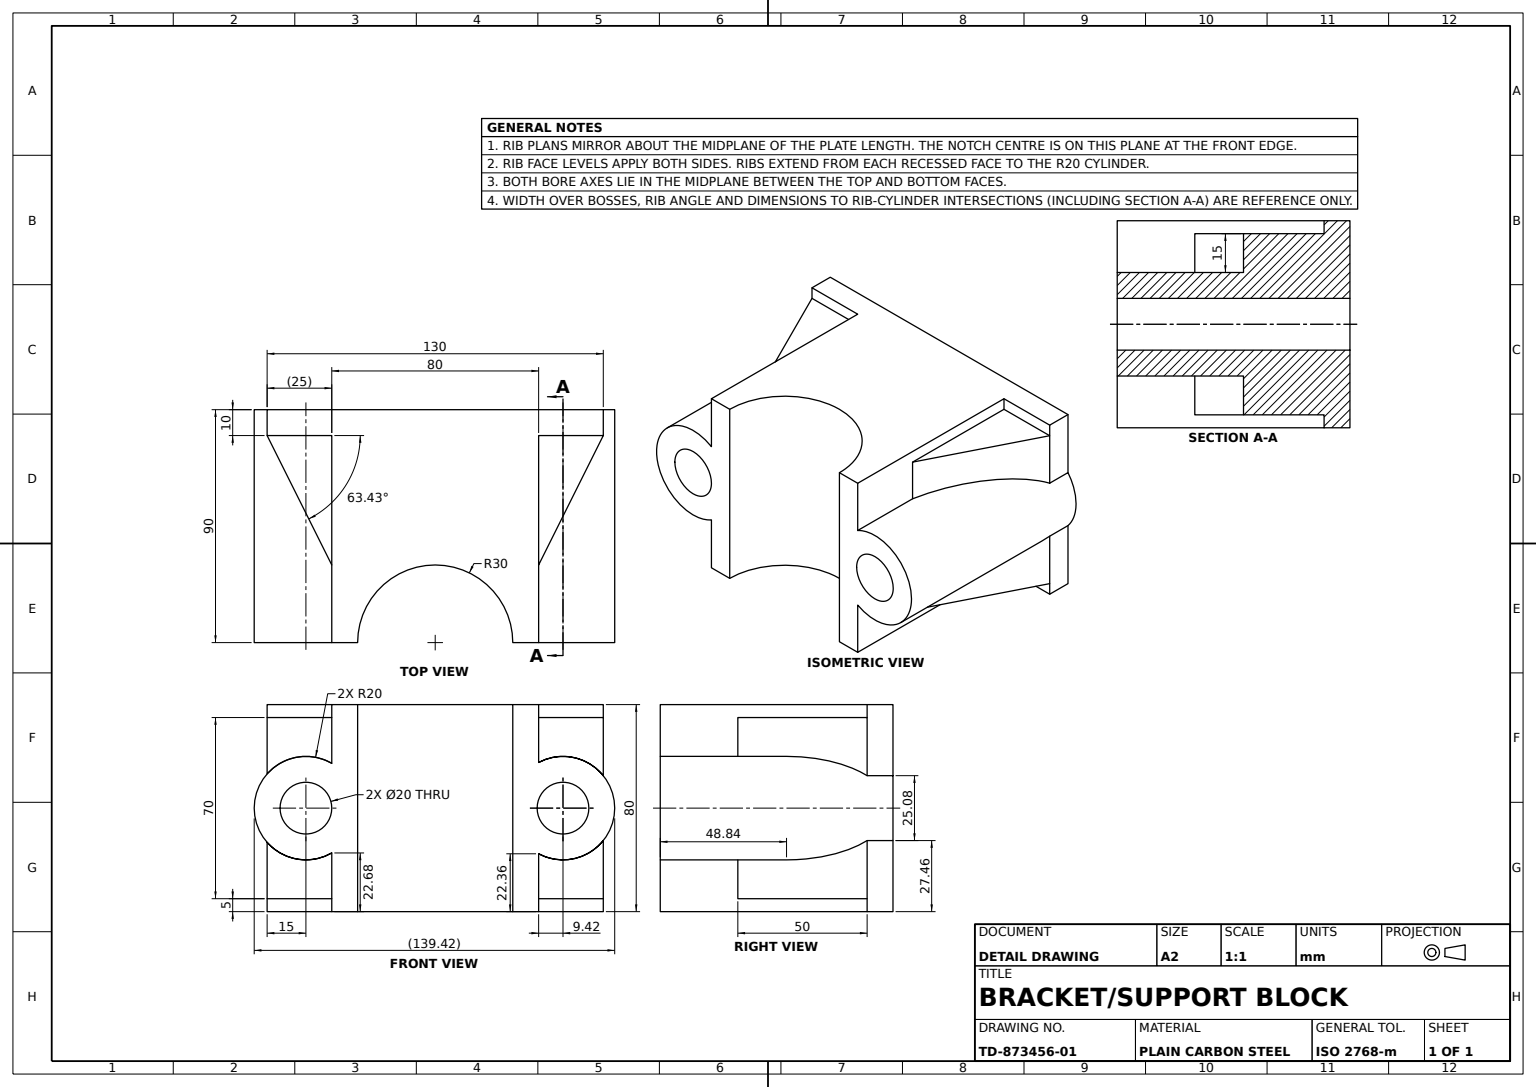
from build123d import *

# Parameters (mm, degrees)
BASE_PLATE_SKETCH_W    = 130
BASE_PLATE_SKETCH_H    = 80
BASE_PLATE_10MM_DEPTH  = 10
MAIN_BODY_PROFILE_W    = 10
MAIN_BODY_PROFILE_H    = 80
MAIN_BODY_DEPTH        = 80
SIDE_WALL_A_DEPTH      = 90
SIDE_WALL_B_DEPTH      = 90
HALF_BORE_SKETCH_R     = 10
HALF_BORE_CUT_DEPTH    = 90
RIB_A_DEPTH            = 28
RIB_B_DEPTH            = 28
BOSS_DEPTH             = 28
RECESS_CUT_A_5MM_DEPTH = 5
RECESS_CUT_B_5MM_DEPTH = 5


with BuildPart() as part:
    # Base Plate Sketch → Base Plate 10mm (new body)
    with BuildSketch(Plane.XY):
        with Locations((65, 40)):
            Rectangle(BASE_PLATE_SKETCH_W, BASE_PLATE_SKETCH_H)
    extrude(amount=BASE_PLATE_10MM_DEPTH)

    # Main Body Profile → Main Body (add)
    with BuildSketch(Plane.XZ):
        with Locations((30, 50)):
            Rectangle(MAIN_BODY_PROFILE_W, MAIN_BODY_PROFILE_H)
        with BuildLine():
            Line((35, 10), (65, 10))
            Line((65, 10), (95, 10))
            Line((95, 10), (95, 90))
            ThreePointArc((95, 90), (65, 60), (35, 90))
            Line((35, 90), (35, 10))
        make_face()
        with Locations((100, 50)):
            Rectangle(MAIN_BODY_PROFILE_W, MAIN_BODY_PROFILE_H)
    extrude(amount=-MAIN_BODY_DEPTH)

    # Side Wall A Sketch → Side Wall A (add)
    with BuildSketch(Plane.XY.offset(90)):
        with BuildLine():
            Line((105, 57.643408065), (105, 22.356591935))
            ThreePointArc((105, 22.356591935), (134.418606683, 40), (105, 57.643408065))
        make_face()
    extrude(amount=-SIDE_WALL_A_DEPTH)

    # Side Wall B Sketch → Side Wall B (add)
    with BuildSketch(Plane.XY.offset(90)):
        with BuildLine():
            Line((25, 57.320508076), (25, 22.679491924))
            ThreePointArc((25, 22.679491924), (-5, 40), (25, 57.320508076))
        make_face()
    extrude(amount=-SIDE_WALL_B_DEPTH)

    # Half Bore Sketch → Half Bore Cut (cut)
    with BuildSketch(Plane.XY.offset(90)):
        with Locations((114.418606683, 40)):
            Circle(HALF_BORE_SKETCH_R)
        with Locations((15, 40)):
            Circle(HALF_BORE_SKETCH_R)
    extrude(amount=-HALF_BORE_CUT_DEPTH, mode=Mode.SUBTRACT)

    # Rib A Sketch → Rib A (add)
    with BuildSketch(Plane.XZ):
        Polygon((105, 10), (105, 60), (130, 10), align=None)
    extrude(amount=-RIB_A_DEPTH)

    # Rib B Sketch → Rib B (add)
    with BuildSketch(Plane.XZ):
        Polygon((25, 10), (25, 60), (0, 10), align=None)
    extrude(amount=-RIB_B_DEPTH)

    # Boss Sketch → Boss (add)
    with BuildSketch(Plane(origin=(0, 80, 0), x_dir=(1, 0, 0), z_dir=(0, 1, 0))):
        Polygon((105, -10), (105, -60), (130, -10), align=None)
        Polygon((25, -10), (25, -60), (0, -10), align=None)
    extrude(amount=-BOSS_DEPTH)

    # Recess A Sketch → Recess Cut A 5mm (cut)
    with BuildSketch(Plane.XZ):
        Polygon((25, 60), (25, 10), (0, 10), align=None)
        Polygon((105, 60), (105, 10), (130, 10), align=None)
    extrude(amount=-RECESS_CUT_A_5MM_DEPTH, mode=Mode.SUBTRACT)

    # Recess B Sketch → Recess Cut B 5mm (cut)
    with BuildSketch(Plane(origin=(0, 80, 0), x_dir=(1, 0, 0), z_dir=(0, 1, 0))):
        Polygon((25, -60), (25, -10), (0, -10), align=None)
        Polygon((105, -60), (105, -10), (130, -10), align=None)
    extrude(amount=-RECESS_CUT_B_5MM_DEPTH, mode=Mode.SUBTRACT)


solid = part.part
